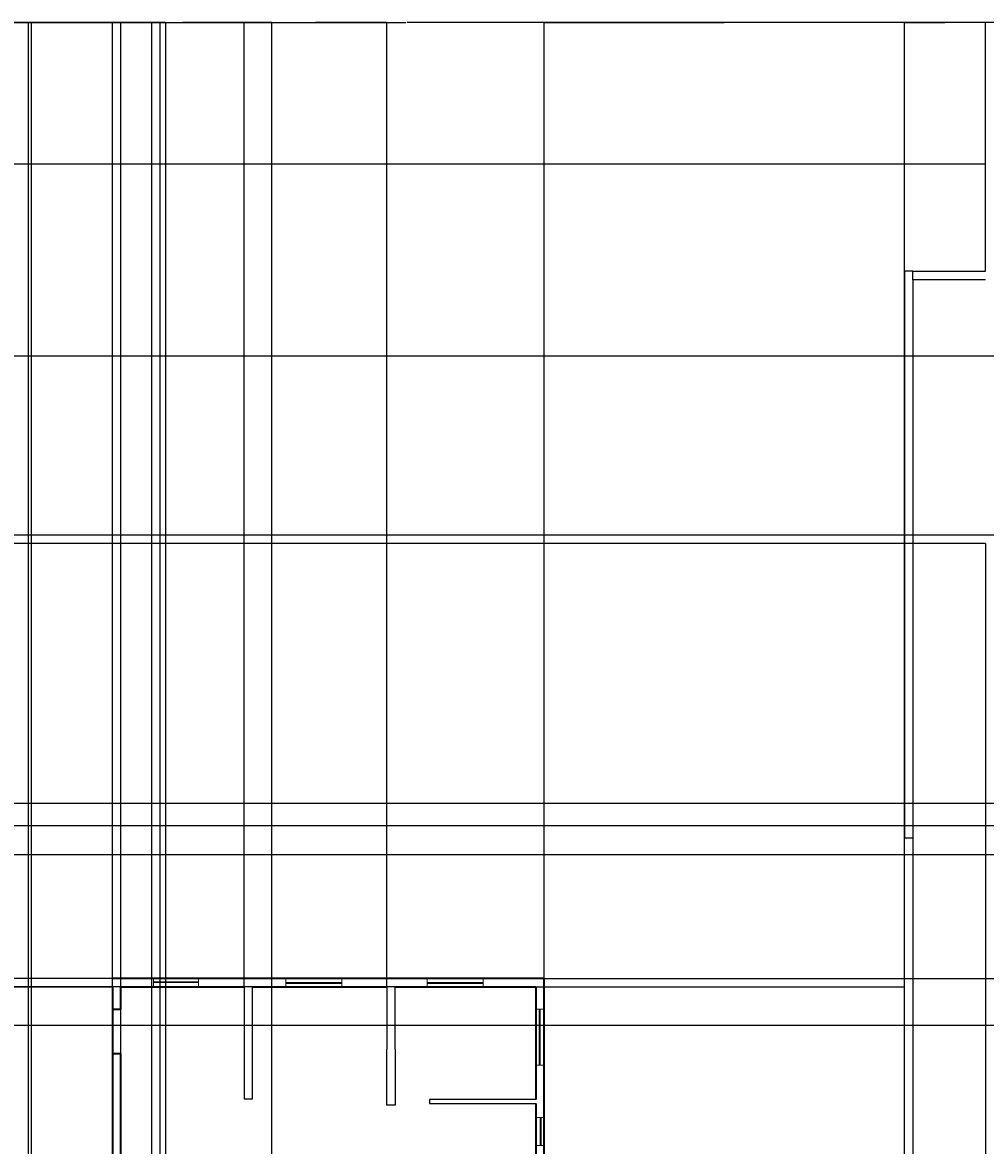
# Model space of a CAD drawing. Units: inches. Extents: x 2029 to 8798, y 1998 to 6373.
# Tile 8 of 11: x 2855 to 3888, y 5168 to 6373. Entities that reach past the tile are written whole.
import ezdxf

# ---------------------------------------------------------------- set-up
doc = ezdxf.new("R2010")
doc.units = ezdxf.units.IN
for name, color, linetype, lineweight in [('A-ANNO-DIMS', 2, 'Continuous', 18), ('A-GLAZ', 4, 'Continuous', 18), ('A-WALL-CIRC', 7, 'Continuous', 25), ('A-WALL-EXTR', 7, 'Continuous', 35), ('A-WALL-INTR', 7, 'Continuous', 25)]:
    doc.layers.add(name, color=color, linetype=linetype, lineweight=lineweight)
doc.styles.get("Standard").update_dxf_attribs({"font": 'arial.ttf'})
doc.dimstyles.get("Standard").update_dxf_attribs({"dimtxt": 0.18, "dimasz": 0.18, "dimexe": 0.18, "dimexo": 0.0625, "dimgap": 0.09, "dimtad": 0, "dimtih": 1, "dimtoh": 1, "dimdec": 4, "dimzin": 0, "dimdsep": 46, "dimtxsty": 'Standard', "dimcen": 0.09, "dimadec": 0, "dimazin": 0, "dimtfac": 1, "dimtdec": 4, "dimtofl": 0, "dimtmove": 0, "dimatfit": 3, "dimfxl": 1, "dimtolj": 1, "dimtzin": 0, "dimarcsym": 0})

# ---------------------------------------------------------------- blocks, each defined once
blk = doc.blocks.new('WIN-60')
for p, q in [((0, 0), (0, 9)), ((0, 4.5), (60, 4.5)), ((0, 3.5), (60, 3.5)), ((60, 9), (60, 0))]:
    blk.add_line(p, q)
blk = doc.blocks.new('WIN-48')
for p, q in [((0, 48), (9, 48)), ((4.5, 48), (4.5, 0)), ((5.5, 48), (5.5, 0)), ((9, 0), (0, 0))]:
    blk.add_line(p, q)
blk = doc.blocks.new('WIN-30')
for p, q in [((0, 0), (0, 9)), ((0, 5.5), (30, 5.5)), ((0, 4.5), (30, 4.5)), ((30, 9), (30, 0))]:
    blk.add_line(p, q)
blk = doc.blocks.new('*D54')
at = {"layer": 'A-ANNO-DIMS', "color": 0, "lineweight": -2, "transparency": 16777216}
for p, q in [((2861.5, 4219.1), (2861.5, 6372.5)), ((2861.7, 6372.4), (2927.3, 6372.4)), ((2993.4, 6372.4), (2927.8, 6372.4)), ((2993.5, 4219.1), (2993.5, 6372.5))]:
    blk.add_line(p, q, dxfattribs=at)
at = {"layer": 'A-ANNO-DIMS', "color": 0, "transparency": 16777216}
for points in [[(2861.7, 6372.4), (2861.7, 6372.3), (2861.5, 6372.4)], [(2993.4, 6372.4), (2993.4, 6372.3), (2993.5, 6372.4)]]:
    blk.add_solid(points, dxfattribs=at)
at = {"layer": 'Defpoints', "color": 0, "transparency": 16777216}
for p in [(2993.5, 6372.4), (2861.5, 4219), (2993.5, 4219)]:
    blk.add_point(p, dxfattribs=at)
at = {"layer": 'A-ANNO-DIMS', "color": 0, "transparency": 16777216, "insert": (2927.5, 6372.4), "char_height": 0.18, "attachment_point": 5}
blk.add_mtext('\\A1;132', dxfattribs=at)
blk = doc.blocks.new('*D55')
at = {"layer": 'A-ANNO-DIMS', "color": 0, "lineweight": -2, "transparency": 16777216}
for p, q in [((3002.5, 4219.1), (3002.5, 6372.5)), ((3002.7, 6372.4), (3062.3, 6372.4)), ((3122.4, 6372.4), (3062.8, 6372.4)), ((3122.5, 4219.1), (3122.5, 6372.5))]:
    blk.add_line(p, q, dxfattribs=at)
at = {"layer": 'A-ANNO-DIMS', "color": 0, "transparency": 16777216}
for points in [[(3002.7, 6372.4), (3002.7, 6372.3), (3002.5, 6372.4)], [(3122.4, 6372.4), (3122.4, 6372.3), (3122.5, 6372.4)]]:
    blk.add_solid(points, dxfattribs=at)
at = {"layer": 'Defpoints', "color": 0, "transparency": 16777216}
for p in [(3122.5, 6372.4), (3002.5, 4219), (3122.5, 4219)]:
    blk.add_point(p, dxfattribs=at)
at = {"layer": 'A-ANNO-DIMS', "color": 0, "transparency": 16777216, "insert": (3062.5, 6372.4), "char_height": 0.18, "attachment_point": 5}
blk.add_mtext('\\A1;120', dxfattribs=at)
blk = doc.blocks.new('*D60')
at = {"layer": 'A-ANNO-DIMS', "color": 0, "lineweight": -2, "transparency": 16777216}
for p, q in [((3414.6, 5347), (4503.7, 5347)), ((4503.5, 5346.8), (4503.5, 5150.7)), ((4503.5, 4954.2), (4503.5, 5150.3)), ((3414.6, 4954), (4503.7, 4954))]:
    blk.add_line(p, q, dxfattribs=at)
at = {"layer": 'A-ANNO-DIMS', "color": 0, "transparency": 16777216}
for points in [[(4503.5, 5346.8), (4503.5, 5346.8), (4503.5, 5347)], [(4503.5, 4954.2), (4503.5, 4954.2), (4503.5, 4954)]]:
    blk.add_solid(points, dxfattribs=at)
at = {"layer": 'Defpoints', "color": 0, "transparency": 16777216}
for p in [(3414.5, 5347), (4503.5, 5347), (3414.5, 4954)]:
    blk.add_point(p, dxfattribs=at)
at = {"layer": 'A-ANNO-DIMS', "color": 0, "transparency": 16777216, "insert": (4503.5, 5150.5), "char_height": 0.18, "attachment_point": 5}
blk.add_mtext('\\A1;393', dxfattribs=at)
blk = doc.blocks.new('*D61')
at = {"layer": 'A-ANNO-DIMS', "color": 0, "lineweight": -2, "transparency": 16777216}
for p, q in [((2732.5, 5347.1), (2732.5, 6372.5)), ((2732.7, 6372.4), (2841.7, 6372.4)), ((2951.3, 6372.4), (2842.3, 6372.4)), ((2951.5, 5347.1), (2951.5, 6372.5))]:
    blk.add_line(p, q, dxfattribs=at)
at = {"layer": 'A-ANNO-DIMS', "color": 0, "transparency": 16777216}
for points in [[(2732.7, 6372.4), (2732.7, 6372.3), (2732.5, 6372.4)], [(2951.3, 6372.4), (2951.3, 6372.3), (2951.5, 6372.4)]]:
    blk.add_solid(points, dxfattribs=at)
at = {"layer": 'Defpoints', "color": 0, "transparency": 16777216}
for p in [(2951.5, 6372.4), (2732.5, 5347), (2951.5, 5347)]:
    blk.add_point(p, dxfattribs=at)
at = {"layer": 'A-ANNO-DIMS', "color": 0, "transparency": 16777216, "insert": (2842, 6372.4), "char_height": 0.18, "attachment_point": 5}
blk.add_mtext('\\A1;219', dxfattribs=at)
blk = doc.blocks.new('*D62')
at = {"layer": 'A-ANNO-DIMS', "color": 0, "lineweight": -2, "transparency": 16777216}
for p, q in [((3414.5, 5347.1), (3414.5, 6372.5)), ((3414.7, 6372.4), (3607.3, 6372.4)), ((3800.6, 6372.4), (3608, 6372.4)), ((3800.8, 5338.1), (3800.8, 6372.5))]:
    blk.add_line(p, q, dxfattribs=at)
at = {"layer": 'A-ANNO-DIMS', "color": 0, "transparency": 16777216}
for points in [[(3414.7, 6372.4), (3414.7, 6372.3), (3414.5, 6372.4)], [(3800.6, 6372.4), (3800.6, 6372.3), (3800.8, 6372.4)]]:
    blk.add_solid(points, dxfattribs=at)
at = {"layer": 'Defpoints', "color": 0, "transparency": 16777216}
for p in [(3800.8, 6372.4), (3414.5, 5347), (3800.8, 5338)]:
    blk.add_point(p, dxfattribs=at)
at = {"layer": 'A-ANNO-DIMS', "color": 0, "transparency": 16777216, "insert": (3607.6, 6372.4), "char_height": 0.18, "attachment_point": 5}
blk.add_mtext('\\A1;386.2', dxfattribs=at)
blk = doc.blocks.new('*D63')
at = {"layer": 'A-ANNO-DIMS', "color": 0, "lineweight": -2, "transparency": 16777216}
for p, q in [((2960.5, 5338.1), (2960.5, 6372.5)), ((2960.7, 6372.4), (3026.2, 6372.4)), ((3092.3, 6372.4), (3026.8, 6372.4)), ((3092.5, 5338.1), (3092.5, 6372.5))]:
    blk.add_line(p, q, dxfattribs=at)
at = {"layer": 'A-ANNO-DIMS', "color": 0, "transparency": 16777216}
for points in [[(2960.7, 6372.4), (2960.7, 6372.3), (2960.5, 6372.4)], [(3092.3, 6372.4), (3092.3, 6372.3), (3092.5, 6372.4)]]:
    blk.add_solid(points, dxfattribs=at)
at = {"layer": 'Defpoints', "color": 0, "transparency": 16777216}
for p in [(3092.5, 6372.4), (2960.5, 5338), (3092.5, 5338)]:
    blk.add_point(p, dxfattribs=at)
at = {"layer": 'A-ANNO-DIMS', "color": 0, "transparency": 16777216, "insert": (3026.5, 6372.4), "char_height": 0.18, "attachment_point": 5}
blk.add_mtext('\\A1;132', dxfattribs=at)
blk = doc.blocks.new('*D64')
at = {"layer": 'A-ANNO-DIMS', "color": 0, "lineweight": -2, "transparency": 16777216}
for p, q in [((3092.5, 5338.1), (3092.5, 6372.5)), ((3092.7, 6372.4), (3168.7, 6372.4)), ((3245.3, 6372.4), (3169.3, 6372.4)), ((3245.5, 5338.1), (3245.5, 6372.5))]:
    blk.add_line(p, q, dxfattribs=at)
at = {"layer": 'A-ANNO-DIMS', "color": 0, "transparency": 16777216}
for points in [[(3092.7, 6372.4), (3092.7, 6372.3), (3092.5, 6372.4)], [(3245.3, 6372.4), (3245.3, 6372.3), (3245.5, 6372.4)]]:
    blk.add_solid(points, dxfattribs=at)
at = {"layer": 'Defpoints', "color": 0, "transparency": 16777216}
for p in [(3245.5, 6372.4), (3092.5, 5338), (3245.5, 5338)]:
    blk.add_point(p, dxfattribs=at)
at = {"layer": 'A-ANNO-DIMS', "color": 0, "transparency": 16777216, "insert": (3169, 6372.4), "char_height": 0.18, "attachment_point": 5}
blk.add_mtext('\\A1;153', dxfattribs=at)
blk = doc.blocks.new('*D65')
at = {"layer": 'A-ANNO-DIMS', "color": 0, "lineweight": -2, "transparency": 16777216}
for p, q in [((3405.5, 5338), (2029.6, 5338)), ((2029.8, 5337.8), (2029.8, 5245.7)), ((2029.8, 5153.2), (2029.8, 5245.3)), ((3405.5, 5153), (2029.6, 5153))]:
    blk.add_line(p, q, dxfattribs=at)
at = {"layer": 'A-ANNO-DIMS', "color": 0, "transparency": 16777216}
for points in [[(2029.8, 5337.8), (2029.8, 5337.8), (2029.8, 5338)], [(2029.8, 5153.2), (2029.8, 5153.2), (2029.8, 5153)]]:
    blk.add_solid(points, dxfattribs=at)
at = {"layer": 'Defpoints', "color": 0, "transparency": 16777216}
for p in [(2029.8, 5338), (3405.5, 5338), (3405.5, 5153)]:
    blk.add_point(p, dxfattribs=at)
at = {"layer": 'A-ANNO-DIMS', "color": 0, "transparency": 16777216, "insert": (2029.8, 5245.5), "char_height": 0.18, "attachment_point": 5}
blk.add_mtext('\\A1;185', dxfattribs=at)
blk = doc.blocks.new('*D70')
at = {"layer": 'A-ANNO-DIMS', "color": 0, "lineweight": -2, "transparency": 16777216}
for p, q in [((3800.8, 6105.7), (3800.8, 6372.5)), ((3800.9, 6372.4), (3844, 6372.4)), ((3887.6, 6372.4), (3844.5, 6372.4)), ((3887.8, 6105.7), (3887.8, 6372.5))]:
    blk.add_line(p, q, dxfattribs=at)
at = {"layer": 'A-ANNO-DIMS', "color": 0, "transparency": 16777216}
for points in [[(3800.9, 6372.4), (3800.9, 6372.3), (3800.8, 6372.4)], [(3887.6, 6372.4), (3887.6, 6372.3), (3887.8, 6372.4)]]:
    blk.add_solid(points, dxfattribs=at)
at = {"layer": 'Defpoints', "color": 0, "transparency": 16777216}
for p in [(3887.8, 6372.4), (3800.8, 6105.6), (3887.8, 6105.6)]:
    blk.add_point(p, dxfattribs=at)
at = {"layer": 'A-ANNO-DIMS', "color": 0, "transparency": 16777216, "insert": (3844.3, 6372.4), "char_height": 0.18, "attachment_point": 5}
blk.add_mtext('\\A1;87', dxfattribs=at)
blk = doc.blocks.new('*D75')
at = {"layer": 'A-ANNO-DIMS', "color": 0, "lineweight": -2, "transparency": 16777216}
for p, q in [((3887.7, 6220.6), (2029.6, 6220.6)), ((2029.8, 6220.4), (2029.8, 6017.3)), ((2029.8, 5813.8), (2029.8, 6016.9)), ((3887.7, 5813.6), (2029.6, 5813.6))]:
    blk.add_line(p, q, dxfattribs=at)
at = {"layer": 'A-ANNO-DIMS', "color": 0, "transparency": 16777216}
for points in [[(2029.8, 6220.4), (2029.8, 6220.4), (2029.8, 6220.6)], [(2029.8, 5813.8), (2029.8, 5813.8), (2029.8, 5813.6)]]:
    blk.add_solid(points, dxfattribs=at)
at = {"layer": 'Defpoints', "color": 0, "transparency": 16777216}
for p in [(2029.8, 6220.6), (3887.8, 6220.6), (3887.8, 5813.6)]:
    blk.add_point(p, dxfattribs=at)
at = {"layer": 'A-ANNO-DIMS', "color": 0, "transparency": 16777216, "insert": (2029.8, 6017.1), "char_height": 0.18, "attachment_point": 5}
blk.add_mtext('\\A1;407', dxfattribs=at)
blk = doc.blocks.new('*D76')
at = {"layer": 'A-ANNO-DIMS', "color": 0, "lineweight": -2, "transparency": 16777216}
for p, q in [((3887.8, 5813.5), (3887.8, 4031.1)), ((4390.8, 5813.5), (4390.8, 4031.1)), ((3887.9, 4031.2), (4139, 4031.2)), ((4390.6, 4031.2), (4139.6, 4031.2))]:
    blk.add_line(p, q, dxfattribs=at)
at = {"layer": 'A-ANNO-DIMS', "color": 0, "transparency": 16777216}
for points in [[(3887.9, 4031.3), (3887.9, 4031.2), (3887.8, 4031.2)], [(4390.6, 4031.3), (4390.6, 4031.2), (4390.8, 4031.2)]]:
    blk.add_solid(points, dxfattribs=at)
at = {"layer": 'Defpoints', "color": 0, "transparency": 16777216}
for p in [(3887.8, 5813.6), (4390.8, 5813.6), (4390.8, 4031.2)]:
    blk.add_point(p, dxfattribs=at)
at = {"layer": 'A-ANNO-DIMS', "color": 0, "transparency": 16777216, "insert": (4139.3, 4031.2), "char_height": 0.18, "attachment_point": 5}
blk.add_mtext('\\A1;503', dxfattribs=at)
blk = doc.blocks.new('*D79')
at = {"layer": 'A-ANNO-DIMS', "color": 0, "lineweight": -2, "transparency": 16777216}
for p, q in [((4043.7, 6014.6), (2029.6, 6014.6)), ((2029.8, 6014.4), (2029.8, 5918.8)), ((2029.8, 5822.8), (2029.8, 5918.4)), ((4043.7, 5822.6), (2029.6, 5822.6))]:
    blk.add_line(p, q, dxfattribs=at)
at = {"layer": 'A-ANNO-DIMS', "color": 0, "transparency": 16777216}
for points in [[(2029.8, 6014.4), (2029.8, 6014.4), (2029.8, 6014.6)], [(2029.8, 5822.8), (2029.8, 5822.8), (2029.8, 5822.6)]]:
    blk.add_solid(points, dxfattribs=at)
at = {"layer": 'Defpoints', "color": 0, "transparency": 16777216}
for p in [(2029.8, 6014.6), (4043.8, 6014.6), (4043.8, 5822.6)]:
    blk.add_point(p, dxfattribs=at)
at = {"layer": 'A-ANNO-DIMS', "color": 0, "transparency": 16777216, "insert": (2029.8, 5918.6), "char_height": 0.18, "attachment_point": 5}
blk.add_mtext('\\A1;192', dxfattribs=at)
blk = doc.blocks.new('*D88')
at = {"layer": 'A-ANNO-DIMS', "color": 0, "lineweight": -2, "transparency": 16777216}
for p, q in [((2142.5, 4445.1), (2142.5, 6372.5)), ((2142.7, 6372.4), (3266.2, 6372.4)), ((4390.6, 6372.4), (3267.1, 6372.4)), ((4390.8, 4574.1), (4390.8, 6372.5))]:
    blk.add_line(p, q, dxfattribs=at)
at = {"layer": 'A-ANNO-DIMS', "color": 0, "transparency": 16777216}
for points in [[(2142.7, 6372.4), (2142.7, 6372.3), (2142.5, 6372.4)], [(4390.6, 6372.4), (4390.6, 6372.3), (4390.8, 6372.4)]]:
    blk.add_solid(points, dxfattribs=at)
at = {"layer": 'Defpoints', "color": 0, "transparency": 16777216}
for p in [(4390.8, 6372.4), (4390.8, 4574), (2142.5, 4445)]:
    blk.add_point(p, dxfattribs=at)
at = {"layer": 'A-ANNO-DIMS', "color": 0, "transparency": 16777216, "insert": (3266.7, 6372.4), "char_height": 0.18, "attachment_point": 5}
blk.add_mtext('\\A1;2248.2', dxfattribs=at)
blk = doc.blocks.new('*D105')
at = {"layer": 'A-ANNO-DIMS', "color": 0, "lineweight": -2, "transparency": 16777216}
for p, q in [((3968.7, 5479.6), (2029.6, 5479.6)), ((2029.8, 5479.4), (2029.8, 5388.3)), ((2029.8, 5296.8), (2029.8, 5387.9)), ((3968.7, 5296.6), (2029.6, 5296.6))]:
    blk.add_line(p, q, dxfattribs=at)
at = {"layer": 'A-ANNO-DIMS', "color": 0, "transparency": 16777216}
for points in [[(2029.8, 5479.4), (2029.8, 5479.4), (2029.8, 5479.6)], [(2029.8, 5296.8), (2029.8, 5296.8), (2029.8, 5296.6)]]:
    blk.add_solid(points, dxfattribs=at)
at = {"layer": 'Defpoints', "color": 0, "transparency": 16777216}
for p in [(2029.8, 5479.6), (3968.8, 5479.6), (3968.8, 5296.6)]:
    blk.add_point(p, dxfattribs=at)
at = {"layer": 'A-ANNO-DIMS', "color": 0, "transparency": 16777216, "insert": (2029.8, 5388.1), "char_height": 0.18, "attachment_point": 5}
blk.add_mtext('\\A1;183', dxfattribs=at)
blk = doc.blocks.new('*D108')
at = {"layer": 'A-ANNO-DIMS', "color": 0, "lineweight": -2, "transparency": 16777216}
for p, q in [((4256.3, 5534.6), (2029.6, 5534.6)), ((2029.8, 5534.4), (2029.8, 5522.8)), ((2029.8, 5510.8), (2029.8, 5522.4)), ((4256.3, 5510.6), (2029.6, 5510.6))]:
    blk.add_line(p, q, dxfattribs=at)
at = {"layer": 'A-ANNO-DIMS', "color": 0, "transparency": 16777216}
for points in [[(2029.8, 5534.4), (2029.8, 5534.4), (2029.8, 5534.6)], [(2029.8, 5510.8), (2029.8, 5510.8), (2029.8, 5510.6)]]:
    blk.add_solid(points, dxfattribs=at)
at = {"layer": 'Defpoints', "color": 0, "transparency": 16777216}
for p in [(4256.4, 5534.6), (2029.8, 5510.6), (4256.4, 5510.6)]:
    blk.add_point(p, dxfattribs=at)
at = {"layer": 'A-ANNO-DIMS', "color": 0, "transparency": 16777216, "insert": (2029.8, 5522.6), "char_height": 0.18, "attachment_point": 5}
blk.add_mtext('\\A1;24', dxfattribs=at)
blk = doc.blocks.new('*D114')
at = {"layer": 'A-ANNO-DIMS', "color": 0, "lineweight": -2, "transparency": 16777216}
for p, q in [((2864.5, 4805.1), (2864.5, 6372.5)), ((2864.7, 6372.4), (2907.8, 6372.4)), ((2951.3, 6372.4), (2908.2, 6372.4)), ((2951.5, 4805.1), (2951.5, 6372.5))]:
    blk.add_line(p, q, dxfattribs=at)
at = {"layer": 'A-ANNO-DIMS', "color": 0, "transparency": 16777216}
for points in [[(2864.7, 6372.4), (2864.7, 6372.3), (2864.5, 6372.4)], [(2951.3, 6372.4), (2951.3, 6372.3), (2951.5, 6372.4)]]:
    blk.add_solid(points, dxfattribs=at)
at = {"layer": 'Defpoints', "color": 0, "transparency": 16777216}
for p in [(2951.5, 6372.4), (2864.5, 4805), (2951.5, 4805)]:
    blk.add_point(p, dxfattribs=at)
at = {"layer": 'A-ANNO-DIMS', "color": 0, "transparency": 16777216, "insert": (2908, 6372.4), "char_height": 0.18, "attachment_point": 5}
blk.add_mtext('\\A1;87', dxfattribs=at)
blk = doc.blocks.new('*D115')
at = {"layer": 'A-ANNO-DIMS', "color": 0, "lineweight": -2, "transparency": 16777216}
for p, q in [((2960.5, 4805.1), (2960.5, 6372.5)), ((2960.7, 6372.4), (2984.3, 6372.4)), ((3008.3, 6372.4), (2984.8, 6372.4)), ((3008.5, 4805.1), (3008.5, 6372.5))]:
    blk.add_line(p, q, dxfattribs=at)
at = {"layer": 'A-ANNO-DIMS', "color": 0, "transparency": 16777216}
for points in [[(2960.7, 6372.4), (2960.7, 6372.3), (2960.5, 6372.4)], [(3008.3, 6372.4), (3008.3, 6372.3), (3008.5, 6372.4)]]:
    blk.add_solid(points, dxfattribs=at)
at = {"layer": 'Defpoints', "color": 0, "transparency": 16777216}
for p in [(3008.5, 6372.4), (2960.5, 4805), (3008.5, 4805)]:
    blk.add_point(p, dxfattribs=at)
at = {"layer": 'A-ANNO-DIMS', "color": 0, "transparency": 16777216, "insert": (2984.5, 6372.4), "char_height": 0.18, "attachment_point": 5}
blk.add_mtext('\\A1;48', dxfattribs=at)

msp = doc.modelspace()

# ---------------------------------------------------------------- linework, layer by layer
at = {"layer": 'A-GLAZ'}
for p, q in [((2995.6043, 5346.9886), (3043.6043, 5346.9886)), ((3137.3124, 5346.9886), (3197.3124, 5346.9886)), ((3288.9212, 5346.9886), (3348.9212, 5346.9886)), ((3414.5292, 5313.9886), (3414.5292, 5253.9886)), ((3414.5292, 5197.8266), (3414.5292, 5167.8266))]:
    msp.add_line(p, q, dxfattribs=at)
at = {"layer": 'A-WALL-CIRC'}
for p, q in [((3809.7657, 6105.6123), (3800.7657, 6105.6123)), ((3800.7657, 6105.6123), (3800.7657, 5497.3491)), ((3809.7657, 6096.6123), (3809.7657, 6105.6123)), ((3809.7657, 6105.6123), (3887.7657, 6105.6123)), ((3887.7657, 6096.6123), (3809.7657, 6096.6123)), ((3809.7657, 6096.6123), (3809.7657, 5497.3826)), ((3809.7657, 5497.3826), (3800.7657, 5497.3826)), ((3800.7657, 5069.4255), (3800.7657, 5497.3491)), ((3809.7657, 5497.3826), (3809.7657, 5069.4255)), ((2951.5292, 5346.9886), (2732.5398, 5346.9886)), ((2732.5398, 5337.9886), (2951.5292, 5337.9886)), ((3405.5292, 5337.9886), (3800.7657, 5337.9886)), ((3414.5292, 5346.9886), (3809.7657, 5346.9886))]:
    msp.add_line(p, q, dxfattribs=at)
at = {"layer": 'A-WALL-EXTR'}
for p, q in [((2960.5292, 5346.9886), (2951.5292, 5346.9886)), ((2951.5292, 5337.9886), (2951.5292, 4962.9886)), ((2951.5292, 5337.9886), (2951.5292, 5313.9886)), ((3414.5292, 5346.9886), (2960.5292, 5346.9886)), ((2960.5292, 5337.9886), (3092.5292, 5337.9886)), ((2960.5292, 5313.9886), (2960.5292, 5337.9886)), ((2960.5292, 5337.9886), (2995.6043, 5337.9886)), ((3101.5292, 5337.9886), (3245.5292, 5337.9886)), ((3101.5292, 5337.9886), (3137.3124, 5337.9886)), ((3254.5292, 5337.9886), (3405.5292, 5337.9886)), ((3254.5292, 5337.9886), (3288.9212, 5337.9886)), ((3405.5292, 5337.9886), (3405.5292, 5216.9886)), ((3405.5292, 5337.9886), (3405.5292, 5313.9886)), ((3414.5292, 5337.9886), (3414.5292, 5346.9886)), ((3414.5292, 4953.9886), (3414.5292, 5337.9886)), ((2951.5292, 5313.9886), (2960.5292, 5313.9886)), ((2960.5292, 5265.9886), (2951.5292, 5265.9886)), ((2960.5292, 5157.9886), (2960.5292, 5265.9886)), ((3405.5292, 5212.9886), (3405.5292, 5152.9886)), ((3405.5292, 5212.9886), (3405.5292, 5197.8266))]:
    msp.add_line(p, q, dxfattribs=at)
at = {"layer": 'A-WALL-INTR'}
for p, q in [((3092.5292, 5337.9886), (3092.5292, 5217.9886)), ((3101.5292, 5217.9886), (3101.5292, 5337.9886)), ((3245.5292, 5337.9886), (3245.5292, 5270.9886)), ((3254.5292, 5270.9886), (3254.5292, 5337.9886)), ((3245.5292, 5211.1527), (3245.5292, 5270.9886)), ((3254.5292, 5270.9886), (3254.5292, 5211.1527)), ((3092.5292, 5217.9886), (3101.5292, 5217.9886)), ((3303.5292, 5216.9886), (3291.5292, 5216.9886)), ((3291.5292, 5216.9886), (3291.5292, 5212.9886)), ((3405.5292, 5216.9886), (3303.5292, 5216.9886)), ((3254.5292, 5211.1527), (3245.5292, 5211.1527)), ((3291.5292, 5212.9886), (3405.5292, 5212.9886))]:
    msp.add_line(p, q, dxfattribs=at)

# ---------------------------------------------------------------- block references
at = {"layer": 'A-GLAZ', "extrusion": (0, 0, -1), "zscale": -1, "rotation": 90}
for name, p in [('WIN-48', (-2995.6043, 5337.9886)), ('WIN-60', (-3405.5292, 5253.9886)), ('WIN-30', (-3405.5292, 5167.8266))]:
    msp.add_blockref(name, p, dxfattribs=at)
at = {"layer": 'A-GLAZ'}
for p in [(3137.3124, 5337.9886), (3288.9212, 5337.9886)]:
    msp.add_blockref('WIN-60', p, dxfattribs=at)

# ---------------------------------------------------------------- dimensions: what is measured, and where the dimension line sits
at = {"layer": 'A-ANNO-DIMS'}
for base, p1, p2, override, picture, middle in [((4390.7657, 6372.3623), (2142.5398, 4444.9886), (4390.7657, 4573.9886), {"dimdec": 1, "dimlfac": 1, "dimrnd": 0, "dimzin": 0, "dimdsep": 46, "dimlunit": 2}, '*D88', (3266.6528, 6372.3623)), ((2951.5292, 6372.3623), (2732.5398, 5346.9886), (2951.5292, 5346.9886), {"dimdec": 0, "dimlfac": 1, "dimrnd": 0, "dimzin": 0, "dimdsep": 46, "dimlunit": 2}, '*D61', (2842.0345, 6372.3623)), ((2993.5398, 6372.3623), (2861.5398, 4218.9886), (2993.5398, 4218.9886), {"dimdec": 0, "dimlfac": 1, "dimrnd": 0, "dimzin": 0, "dimdsep": 46, "dimlunit": 2}, '*D54', (2927.5398, 6372.3623)), ((2951.5292, 6372.3623), (2864.5292, 4804.9886), (2951.5292, 4804.9886), {"dimdec": 0, "dimlfac": 1, "dimrnd": 0, "dimzin": 0, "dimdsep": 46, "dimlunit": 2}, '*D114', (2908.0292, 6372.3623)), ((3092.5292, 6372.3623), (2960.5292, 5337.9886), (3092.5292, 5337.9886), {"dimdec": 0, "dimlfac": 1, "dimrnd": 0, "dimzin": 0, "dimdsep": 46, "dimlunit": 2}, '*D63', (3026.5292, 6372.3623)), ((3008.5292, 6372.3623), (2960.5292, 4804.9886), (3008.5292, 4804.9886), {"dimdec": 0, "dimlfac": 1, "dimrnd": 0, "dimzin": 0, "dimdsep": 46, "dimlunit": 2}, '*D115', (2984.5292, 6372.3623)), ((3122.5398, 6372.3623), (3002.5398, 4218.9886), (3122.5398, 4218.9886), {"dimdec": 0, "dimlfac": 1, "dimrnd": 0, "dimzin": 0, "dimdsep": 46, "dimlunit": 2}, '*D55', (3062.5398, 6372.3623)), ((3245.5292, 6372.3623), (3092.5292, 5337.9886), (3245.5292, 5337.9886), {"dimdec": 0, "dimlfac": 1, "dimrnd": 0, "dimzin": 0, "dimdsep": 46, "dimlunit": 2}, '*D64', (3169.0292, 6372.3623)), ((3800.7657, 6372.3623), (3414.5292, 5346.9886), (3800.7657, 5337.9886), {"dimdec": 1, "dimlfac": 1, "dimrnd": 0, "dimzin": 0, "dimdsep": 46, "dimlunit": 2}, '*D62', (3607.6475, 6372.3623)), ((3887.7657, 6372.3623), (3800.7657, 6105.6123), (3887.7657, 6105.6123), {"dimdec": 0, "dimlfac": 1, "dimrnd": 0, "dimzin": 0, "dimdsep": 46, "dimlunit": 2}, '*D70', (3844.2657, 6372.3623)), ((4390.7657, 4031.2386), (3887.7657, 5813.6123), (4390.7657, 5813.6123), {"dimdec": 0, "dimlfac": 1, "dimrnd": 0, "dimzin": 0, "dimdsep": 46, "dimlunit": 2}, '*D76', (4139.2657, 4031.2386))]:
    dim = msp.add_linear_dim(base=base, p1=p1, p2=p2, dimstyle='Standard', override=override, dxfattribs=at)
    dim.commit()
    dim.dimension.update_dxf_attribs({"geometry": picture, "text_midpoint": middle})
for base, p1, p2, picture, middle in [((2029.7898, 6220.6123), (3887.7657, 5813.6123), (3887.7657, 6220.6123), '*D75', (2029.7898, 6017.1123)), ((2029.7898, 6014.6123), (4043.7657, 5822.6123), (4043.7657, 6014.6123), '*D79', (2029.7898, 5918.6123)), ((2029.7898, 5510.6123), (4256.3869, 5534.6123), (4256.3869, 5510.6123), '*D108', (2029.7898, 5522.6123)), ((2029.7898, 5479.6123), (3968.7657, 5296.6123), (3968.7657, 5479.6123), '*D105', (2029.7898, 5388.1123)), ((2029.7898, 5337.9886), (3405.5292, 5152.9886), (3405.5292, 5337.9886), '*D65', (2029.7898, 5245.4886)), ((4503.5157, 5346.9886), (3414.5292, 4953.9886), (3414.5292, 5346.9886), '*D60', (4503.5157, 5150.4886))]:
    dim = msp.add_linear_dim(base=base, p1=p1, p2=p2, angle=90, dimstyle='Standard', override={"dimdec": 0, "dimlfac": 1, "dimrnd": 0, "dimzin": 0, "dimdsep": 46, "dimlunit": 2}, dxfattribs=at)
    dim.commit()
    dim.dimension.update_dxf_attribs({"geometry": picture, "text_midpoint": middle})

doc.saveas('drawing.dxf')
